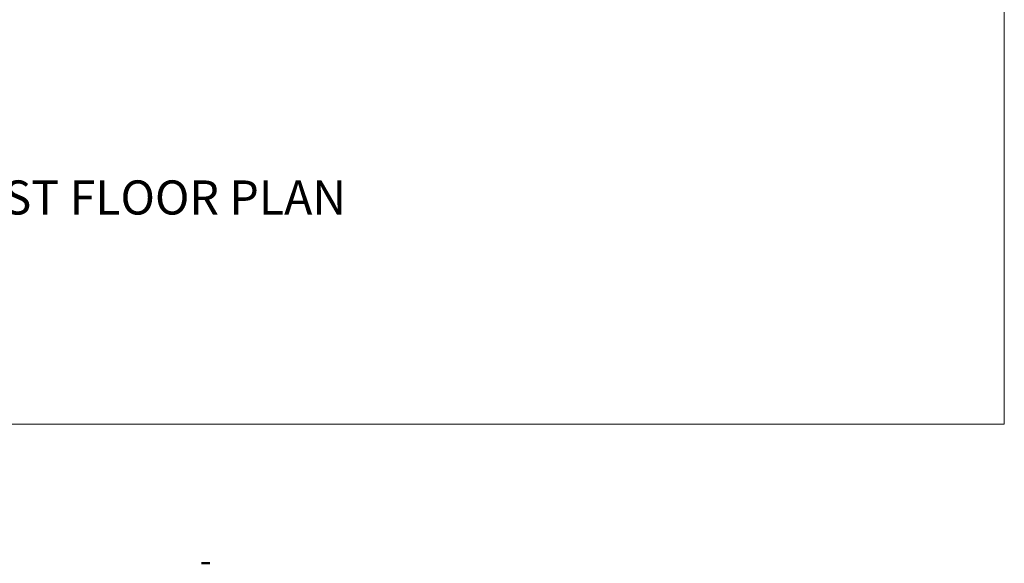
# Model space of a CAD drawing. Units: inches. Extents: x 1901 to 2863, y 888 to 2433.
# Tile 21 of 91: x 2343 to 2863, y 888 to 1175. Entities that reach past the tile are written whole.
import ezdxf

# ---------------------------------------------------------------- set-up
doc = ezdxf.new("R2010")
doc.units = ezdxf.units.IN
for name, color, linetype, lineweight in [('A-ANNO-TEXT', 7, 'Continuous', 35), ('A-FLOR-FIXT', 9, 'Continuous', 18), ('A-WALL', 7, 'Continuous', 50), ('A-WALL-PATT', 8, 'Continuous', 13)]:
    doc.layers.add(name, color=color, linetype=linetype, lineweight=lineweight)
doc.styles.get("Standard").update_dxf_attribs({"font": 'arial.ttf'})

msp = doc.modelspace()

# ---------------------------------------------------------------- hatches: boundary and pattern name
at = {"layer": 'A-WALL-PATT'}
h = msp.add_hatch(dxfattribs=at)
h.set_pattern_fill('ANSI32', color=256)
h.paths.add_polyline_path([(2192.5, 2274.13), (2141.26, 2274.13), (2141.26, 2269.63), (2192.5, 2269.63)])
h.paths.add_polyline_path([(2259.93, 2274.13), (2216.5, 2274.13), (2216.5, 2269.63), (2255.43, 2269.63), (2255.43, 2214.63), (2250.81, 2214.63), (2250.81, 2210.13), (2259.93, 2210.13), (2259.93, 2215.13), (2271.76, 2215.13), (2271.76, 2217.38), (2271.76, 2219.63), (2259.93, 2219.63)])
h.paths.add_polyline_path([(2171.43, 2269.63), (2166.93, 2269.63), (2166.93, 2219.63), (2121.24, 2219.63), (2121.24, 2215.13), (2166.93, 2215.13), (2166.93, 2083.13), (2161.81, 2083.13), (2161.81, 2078.63), (2171.43, 2078.63), (2177, 2078.63), (2177, 2080.88), (2177, 2083.13), (2171.43, 2083.13), (2171.43, 2210.13), (2230.91, 2210.13), (2230.91, 2212.38), (2230.91, 2214.63), (2171.43, 2214.63)])
h.paths.add_polyline_path([(2117.26, 2274.13), (2089.43, 2274.13), (2089.43, 2219.63), (2081.14, 2219.63), (2081.14, 2215.13), (2089.43, 2215.13), (2098, 2215.13), (2098, 2217.38), (2098, 2219.63), (2093.93, 2219.63), (2093.93, 2269.63), (2117.26, 2269.63), (2117.26, 2271.88)])
h.paths.add_polyline_path([(2343.43, 2219.63), (2329.29, 2219.63), (2329.29, 2215.13), (2338.93, 2215.13), (2338.93, 2184.74), (2343.43, 2184.74)])
h.paths.add_polyline_path([(2338.93, 2083.13), (2329.29, 2083.13), (2208.97, 2083.13), (2208.97, 2078.63), (2338.93, 2078.63)])
h.paths.add_polyline_path([(2343.43, 2136.74), (2338.93, 2136.74), (2338.93, 1872.63), (2343.43, 1872.63)])
h.paths.add_polyline_path([(2343.43, 1863.63), (2397.68, 1863.63), (2397.68, 1821.63), (2384.14, 1821.63), (2384.14, 1812.63), (2418.33, 1812.63), (2418.33, 1817.13), (2418.33, 1821.63), (2406.68, 1821.63), (2406.68, 1863.63), (2459.5, 1863.63), (2459.5, 1821.63), (2447.14, 1821.63), (2447.14, 1812.63), (2459.5, 1812.63), (2468.5, 1812.63), (2468.5, 1872.63), (2394.43, 1872.63), (2334.43, 1872.63), (2334.43, 1812.63), (2343.43, 1812.63), (2353.25, 1812.63), (2353.25, 1821.63), (2343.43, 1821.63)])
h.paths.add_polyline_path([(2510.01, 1872.63), (2468.5, 1872.63), (2468.5, 1868.13), (2510.01, 1868.13)])
h.paths.add_polyline_path([(2514.01, 1817.13), (2468.5, 1817.13), (2468.5, 1812.63), (2482.11, 1812.63), (2482.11, 1800.61), (2486.61, 1800.61), (2486.61, 1812.63), (2514.01, 1812.63)])
h.paths.add_polyline_path([(2299.25, 1814.88), (2299.25, 1817.13), (2295.93, 1817.13), (2295.93, 1854.17), (2293.68, 1854.17), (2291.43, 1854.17), (2291.43, 1817.13), (2266.11, 1817.13), (2266.11, 1812.63), (2299.25, 1812.63)])
h.paths.add_polyline_path([(2218.11, 1817.13), (2206.46, 1817.13), (2171.43, 1817.13), (2171.43, 1949.13), (2190.1, 1949.13), (2190.1, 1953.63), (2163.47, 1953.63), (2163.47, 1949.13), (2166.93, 1949.13), (2166.93, 1817.13), (2114.3, 1817.13), (2114.3, 1812.63), (2218.11, 1812.63)])
h.paths.add_polyline_path([(2029.43, 1970.92), (2024.93, 1970.92), (2024.93, 1912.72), (2029.43, 1912.72)])
h.paths.add_polyline_path([(2132.3, 1953.63), (2113.93, 1953.63), (2113.93, 1975.89), (2111.68, 1975.89), (2109.43, 1975.89), (2109.43, 1953.63), (2029.43, 1953.63), (2029.43, 1949.13), (2132.3, 1949.13)])
h.paths.add_polyline_path([(2029.43, 1853.61), (2029.31, 1853.61), (2029.31, 1853.61), (2029.43, 1853.61), (2029.43, 1864.72), (2024.93, 1864.72), (2024.93, 1812.63), (2066.3, 1812.63), (2066.3, 1814.88), (2066.3, 1817.13), (2029.43, 1817.13)])
h.paths.add_polyline_path([(2122.93, 2010.09), (2120.68, 2010.09), (2118.43, 2010.09), (2118.43, 2006.13), (2029.43, 2006.13), (2029.43, 2001.63), (2109.43, 2001.63), (2109.43, 1998.04), (2113.93, 1998.04), (2113.93, 2001.63), (2122.93, 2001.63)])
h.paths.add_polyline_path([(2029.43, 2031.38), (2024.93, 2031.38), (2024.93, 1994.92), (2027.18, 1994.92), (2029.43, 1994.92)])
h.paths.add_polyline_path([(2029.43, 2136.74), (2024.93, 2136.74), (2024.93, 2067.38), (2027.18, 2067.38), (2029.43, 2067.38)])
h.paths.add_polyline_path([(2125.62, 2083.13), (2029.43, 2083.13), (2029.43, 2078.63), (2118.43, 2078.63), (2118.43, 2030.71), (2122.93, 2030.71), (2122.93, 2078.63), (2125.62, 2078.63)])
h.paths.add_polyline_path([(2029.43, 2215.13), (2040.47, 2215.13), (2040.47, 2217.38), (2040.47, 2219.63), (2024.93, 2219.63), (2024.93, 2184.74), (2029.43, 2184.74), (2029.43, 2187.78)])
h.paths.add_polyline_path([(2686.43, 2274.13), (2659.28, 2274.13), (2659.28, 2269.63), (2681.93, 2269.63), (2681.93, 2219.63), (2676.82, 2219.63), (2676.82, 2215.13), (2681.93, 2215.13), (2697.01, 2215.13), (2697.01, 2217.38), (2697.01, 2219.63), (2686.43, 2219.63)])
h.paths.add_polyline_path([(2609.93, 2269.63), (2635.28, 2269.63), (2635.28, 2274.13), (2571.43, 2274.13), (2571.43, 2269.63), (2605.43, 2269.63), (2605.43, 2214.63), (2549.1, 2214.63), (2549.1, 2210.13), (2605.43, 2210.13), (2605.43, 2083.13), (2601.01, 2083.13), (2601.01, 2080.88), (2601.01, 2078.63), (2609.93, 2078.63), (2616.16, 2078.63), (2616.16, 2080.88), (2616.16, 2083.13), (2609.93, 2083.13), (2609.93, 2215.13), (2651.46, 2215.13), (2651.46, 2217.38), (2651.46, 2219.63), (2609.93, 2219.63)])
h.paths.add_polyline_path([(2521.43, 2269.63), (2547.43, 2269.63), (2547.43, 2271.88), (2547.43, 2274.13), (2516.93, 2274.13), (2516.93, 2219.63), (2506.41, 2219.63), (2506.41, 2215.13), (2516.93, 2215.13), (2516.93, 2210.13), (2525.4, 2210.13), (2525.4, 2212.38), (2525.4, 2214.63), (2521.43, 2214.63)])
h.paths.add_polyline_path([(2456.01, 2219.63), (2439.43, 2219.63), (2439.43, 2187.89), (2443.93, 2187.89), (2443.93, 2215.13), (2456.01, 2215.13)])
h.paths.add_polyline_path([(2752.93, 2219.63), (2739.48, 2219.63), (2739.48, 2215.13), (2748.43, 2215.13), (2748.43, 2187.89), (2752.93, 2187.89)])
h.paths.add_polyline_path([(2752.93, 2139.89), (2748.43, 2139.89), (2748.43, 2083.13), (2648.42, 2083.13), (2648.42, 2078.63), (2654.93, 2078.63), (2654.93, 2039.44), (2659.43, 2039.44), (2659.43, 2078.63), (2748.43, 2078.63), (2748.43, 2063.43), (2752.93, 2063.43)])
h.paths.add_polyline_path([(2752.93, 2010.63), (2659.43, 2010.63), (2659.43, 2015.65), (2654.93, 2015.65), (2654.93, 2010.63), (2605.43, 2010.63), (2605.43, 1920.97), (2609.93, 1920.97), (2609.93, 2006.13), (2748.43, 2006.13), (2748.43, 1982.47), (2752.93, 1982.47)])
h.paths.add_polyline_path([(2752.93, 2027.43), (2748.43, 2027.43), (2748.43, 2010.63), (2752.93, 2010.63)])
h.paths.add_polyline_path([(2748.43, 1886.13), (2609.93, 1886.13), (2609.93, 1889.72), (2605.43, 1889.72), (2605.43, 1861.26), (2609.93, 1861.26), (2609.93, 1881.63), (2748.43, 1881.63)])
h.paths.add_polyline_path([(2456.86, 2228.83), (2498.4, 2228.83), (2498.4, 2247.49), (2456.86, 2247.49)], flags=9)
h.paths.add_polyline_path([(2038.6, 2237.42), (2080.17, 2237.42), (2080.17, 2256.08), (2038.6, 2256.08)], flags=9)
h.paths.add_polyline_path([(2292.01, 1062.39), (2539.93, 1062.39), (2539.93, 1099.49), (2292.01, 1099.49)], flags=9)
h.paths.add_polyline_path([(2424.91, 1832.25), (2448.51, 1832.25), (2448.51, 1846.68), (2424.91, 1846.68)], flags=25)
h.paths.add_polyline_path([(2359.08, 1832.25), (2382.68, 1832.25), (2382.68, 1846.68), (2359.08, 1846.68)], flags=25)
h.paths.add_polyline_path([(2352.9, 1684.8), (2367.54, 1684.8), (2367.54, 1697.17), (2352.9, 1697.17)], flags=9)
h.paths.add_polyline_path([(2079.29, 1755.83), (2169.02, 1755.83), (2169.02, 1774.37), (2079.29, 1774.37)], flags=9)
h.paths.add_polyline_path([(2404.09, 1373.86), (2404.09, 1463.59), (2385.54, 1463.59), (2385.54, 1373.86)], flags=9)
h.paths.add_polyline_path([(2268.09, 2236.37), (2309.64, 2236.37), (2309.64, 2255.03), (2268.09, 2255.03)], flags=9)
h.paths.add_polyline_path([(2575.96, 1700.95), (2665.7, 1700.95), (2665.7, 1719.5), (2575.96, 1719.5)], flags=9)
h.paths.add_polyline_path([(2302.96, 1878.47), (2329.52, 1878.47), (2329.52, 1888.78), (2302.96, 1888.78)], flags=9)
h.paths.add_polyline_path([(2097.42, 2240.58), (2126.57, 2240.58), (2126.57, 2259.23), (2097.42, 2259.23)], flags=9)
h.paths.add_polyline_path([(2208.72, 2246.12), (2237.88, 2246.12), (2237.88, 2264.78), (2208.72, 2264.78)], flags=9)
h.paths.add_polyline_path([(2038.15, 1925.96), (2076.99, 1925.96), (2076.99, 1944.62), (2038.15, 1944.62)], flags=9)
h.paths.add_polyline_path([(2239.14, 1926.67), (2288.46, 1926.67), (2288.46, 1945.33), (2239.14, 1945.33)], flags=9)
h.paths.add_polyline_path([(2175.43, 2007.33), (2212.36, 2007.33), (2212.36, 2025.99), (2175.43, 2025.99)], flags=9)
h.paths.add_polyline_path([(2225.03, 2091.79), (2263.87, 2091.79), (2263.87, 2110.45), (2225.03, 2110.45)], flags=9)
h.paths.add_polyline_path([(2035.4, 2098.48), (2074.24, 2098.48), (2074.24, 2117.14), (2035.4, 2117.14)], flags=9)
h.paths.add_polyline_path([(2050.1, 2029.21), (2083.26, 2029.21), (2083.26, 2047.87), (2050.1, 2047.87)], flags=9)
h.paths.add_polyline_path([(2069.68, 1956.72), (2098.83, 1956.72), (2098.83, 1975.38), (2069.68, 1975.38)], flags=25)
h.paths.add_polyline_path([(2328.62, 1753.34), (2361.66, 1753.34), (2361.66, 1771.99), (2328.62, 1771.99)], flags=9)
h.paths.add_polyline_path([(2395.16, 2060.89), (2395.16, 2140.65), (2378.68, 2140.65), (2378.68, 2060.89)], flags=9)
h.paths.add_polyline_path([(2463.73, 2059.02), (2492.89, 2059.02), (2492.89, 2077.68), (2463.73, 2077.68)], flags=9)
h.paths.add_polyline_path([(2458.03, 2181.54), (2496.87, 2181.54), (2496.87, 2200.19), (2458.03, 2200.19)], flags=9)
h.paths.add_polyline_path([(2527.58, 2243.07), (2556.73, 2243.07), (2556.73, 2261.73), (2527.58, 2261.73)], flags=9)
h.paths.add_polyline_path([(2694.46, 2232.77), (2736.03, 2232.77), (2736.03, 2251.42), (2694.46, 2251.42)], flags=9)
h.paths.add_polyline_path([(2637.82, 2249.22), (2666.98, 2249.22), (2666.98, 2267.88), (2637.82, 2267.88)], flags=9)
h.paths.add_polyline_path([(2623.69, 2183.54), (2662.53, 2183.54), (2662.53, 2202.2), (2623.69, 2202.2)], flags=9)
h.paths.add_polyline_path([(2691.97, 2021.5), (2725.12, 2021.5), (2725.12, 2040.16), (2691.97, 2040.16)], flags=9)
h.paths.add_polyline_path([(2621.04, 1975.91), (2662.34, 1975.91), (2662.34, 1994.57), (2621.04, 1994.57)], flags=25)
h.paths.add_polyline_path([(2479.03, 1927.62), (2519.84, 1927.62), (2519.84, 1946.28), (2479.03, 1946.28)], flags=9)
h.paths.add_polyline_path([(2670.94, 1849.08), (2716.01, 1849.08), (2716.01, 1867.73), (2670.94, 1867.73)], flags=9)
h.paths.add_polyline_path([(2523.61, 1782.96), (2550.17, 1782.96), (2550.17, 1793.26), (2523.61, 1793.26)], flags=9)
h.paths.add_polyline_path([(2450.84, 1207.33), (2492.39, 1207.33), (2492.39, 1225.99), (2450.84, 1225.99)], flags=9)
h.paths.add_polyline_path([(2527.75, 1203.84), (2556.91, 1203.84), (2556.91, 1222.5), (2527.75, 1222.5)], flags=9)
h.paths.add_polyline_path([(2639.11, 1207.2), (2668.27, 1207.2), (2668.27, 1225.86), (2639.11, 1225.86)], flags=9)
h.paths.add_polyline_path([(2692.59, 1218.97), (2734.17, 1218.97), (2734.17, 1237.62), (2692.59, 1237.62)], flags=9)
h.paths.add_polyline_path([(2669.27, 1366.33), (2708.11, 1366.33), (2708.11, 1384.99), (2669.27, 1384.99)], flags=9)
h.paths.add_polyline_path([(2463.31, 1358.03), (2502.15, 1358.03), (2502.15, 1376.69), (2463.31, 1376.69)], flags=9)
h.paths.add_polyline_path([(2494.72, 1449.96), (2531.65, 1449.96), (2531.65, 1468.62), (2494.72, 1468.62)], flags=9)
h.paths.add_polyline_path([(2675.57, 1422.16), (2708.72, 1422.16), (2708.72, 1440.81), (2675.57, 1440.81)], flags=9)
h.paths.add_polyline_path([(2685.63, 1493.89), (2714.79, 1493.89), (2714.79, 1512.55), (2685.63, 1512.55)], flags=9)
h.paths.add_polyline_path([(2686.8, 1529.91), (2725.65, 1529.91), (2725.65, 1548.57), (2686.8, 1548.57)], flags=9)
h.paths.add_polyline_path([(2503.65, 1537.99), (2552.97, 1537.99), (2552.97, 1556.65), (2503.65, 1556.65)], flags=9)
h.paths.add_polyline_path([(2291.71, 1643.5), (2318.28, 1643.5), (2318.28, 1653.81), (2291.71, 1653.81)], flags=9)
h.paths.add_polyline_path([(2450.63, 1610.52), (2477.19, 1610.52), (2477.19, 1620.82), (2450.63, 1620.82)], flags=9)
h.paths.add_polyline_path([(2359.99, 1551.81), (2422.25, 1551.81), (2422.25, 1562.12), (2359.99, 1562.12)], flags=9)
h.paths.add_polyline_path([(2280.11, 1249.01), (2321.65, 1249.01), (2321.65, 1267.66), (2280.11, 1267.66)], flags=9)
h.paths.add_polyline_path([(2164.06, 1274.23), (2193.22, 1274.23), (2193.22, 1292.89), (2164.06, 1292.89)], flags=9)
h.paths.add_polyline_path([(2118.21, 1277.69), (2151.25, 1277.69), (2151.25, 1296.35), (2118.21, 1296.35)], flags=9)
h.paths.add_polyline_path([(2031.95, 1268.53), (2073.52, 1268.53), (2073.52, 1287.19), (2031.95, 1287.19)], flags=9)
h.paths.add_polyline_path([(2050.2, 1409.08), (2089.04, 1409.08), (2089.04, 1427.74), (2050.2, 1427.74)], flags=9)
h.paths.add_polyline_path([(2243.74, 1421.03), (2282.58, 1421.03), (2282.58, 1439.69), (2243.74, 1439.69)], flags=9)
h.paths.add_polyline_path([(2190.75, 1509.77), (2231.56, 1509.77), (2231.56, 1528.43), (2190.75, 1528.43)], flags=9)
h.paths.add_polyline_path([(2058.39, 1475.42), (2091.55, 1475.42), (2091.55, 1494.07), (2058.39, 1494.07)], flags=9)
h.paths.add_polyline_path([(2062.45, 1553.09), (2091.6, 1553.09), (2091.6, 1571.75), (2062.45, 1571.75)], flags=9)
h.paths.add_polyline_path([(2219.52, 1590.37), (2266.15, 1590.37), (2266.15, 1609.02), (2219.52, 1609.02)], flags=9)
h.paths.add_polyline_path([(2041.07, 1584.19), (2079.91, 1584.19), (2079.91, 1602.85), (2041.07, 1602.85)], flags=9)
h = msp.add_hatch(dxfattribs=at)
h.set_pattern_fill('ANSI32', color=256)
h.paths.add_polyline_path([(2443.93, 2139.89), (2439.43, 2139.89), (2439.43, 2069.35), (2441.68, 2069.35), (2443.93, 2069.35), (2443.93, 2078.63), (2521.93, 2078.63), (2521.93, 2075.07), (2524.18, 2075.07), (2526.43, 2075.07), (2526.43, 2078.63), (2571.75, 2078.63), (2571.75, 2080.88), (2571.75, 2083.13), (2443.93, 2083.13)])
h.paths.add_polyline_path([(2526.43, 2054.63), (2524.18, 2054.63), (2521.93, 2054.63), (2521.93, 2030.63), (2443.93, 2030.63), (2443.93, 2045.35), (2439.43, 2045.35), (2439.43, 1983.87), (2443.93, 1983.87), (2443.93, 2026.13), (2521.93, 2026.13), (2526.43, 2026.13)])
h.paths.add_polyline_path([(2443.93, 1923.87), (2439.43, 1923.87), (2439.43, 1872.63), (2443.93, 1872.63)])
h.paths.add_polyline_path([(2636.23, 1766.13), (2609.93, 1766.13), (2609.93, 1779.79), (2605.43, 1779.79), (2605.43, 1766.13), (2486.61, 1766.13), (2486.61, 1770.67), (2482.11, 1770.67), (2482.11, 1766.13), (2482.11, 1761.63), (2636.23, 1761.63), (2636.23, 1763.88)])
h.paths.add_polyline_path([(2519.54, 1663.38), (2519.54, 1665.63), (2494.93, 1665.63), (2481.83, 1665.63), (2481.83, 1663.38), (2481.83, 1661.13), (2490.43, 1661.13), (2490.43, 1640.16), (2494.93, 1640.16), (2494.93, 1661.13), (2519.54, 1661.13)])
h.paths.add_polyline_path([(2443.93, 1712.13), (2443.93, 1716.63), (2414.46, 1716.63), (2414.46, 1712.13), (2439.43, 1712.13), (2439.43, 1545.51), (2443.93, 1545.51), (2443.93, 1661.13), (2448.47, 1661.13), (2448.47, 1665.63), (2443.93, 1665.63)])
h.paths.add_polyline_path([(2343.43, 1712.13), (2365.52, 1712.13), (2365.52, 1714.38), (2365.52, 1716.63), (2333.87, 1716.63), (2333.87, 1714.38), (2333.87, 1712.13), (2338.93, 1712.13), (2338.93, 1575.63), (2338.93, 1545.51), (2343.43, 1545.51), (2343.43, 1547.51), (2343.43, 1580.13)])
h.paths.add_polyline_path([(2752.93, 1665.63), (2579.54, 1665.63), (2579.54, 1661.13), (2615.93, 1661.13), (2615.93, 1529.13), (2598.93, 1529.13), (2598.93, 1524.63), (2623.13, 1524.63), (2623.13, 1526.88), (2623.13, 1529.13), (2620.43, 1529.13), (2620.43, 1661.13), (2748.43, 1661.13), (2748.43, 1633.5), (2752.93, 1633.5)])
h.paths.add_polyline_path([(2752.93, 1419.93), (2748.43, 1419.93), (2748.43, 1400.13), (2659.43, 1400.13), (2659.43, 1444.33), (2657.18, 1444.33), (2654.93, 1444.33), (2654.93, 1400.13), (2643.65, 1400.13), (2643.65, 1395.63), (2748.43, 1395.63), (2748.43, 1364.04), (2752.93, 1364.04)])
h.paths.add_polyline_path([(2752.93, 1492.88), (2748.43, 1492.88), (2748.43, 1476.63), (2667.43, 1476.63), (2667.43, 1479.71), (2665.18, 1479.71), (2662.93, 1479.71), (2662.93, 1476.63), (2654.93, 1476.63), (2654.93, 1469.54), (2659.43, 1469.54), (2659.43, 1472.13), (2748.43, 1472.13), (2748.43, 1455.93), (2752.93, 1455.93)])
h.paths.add_polyline_path([(2752.93, 1304.04), (2748.43, 1304.04), (2748.43, 1263.63), (2738.66, 1263.63), (2738.66, 1259.13), (2752.93, 1259.13)])
h.paths.add_polyline_path([(2685.93, 1259.13), (2695.49, 1259.13), (2695.49, 1261.38), (2695.49, 1263.63), (2677.84, 1263.63), (2677.84, 1261.38), (2677.84, 1259.13), (2681.43, 1259.13), (2681.43, 1203.63), (2653.28, 1203.63), (2653.28, 1199.13), (2685.93, 1199.13), (2685.93, 1203.63)])
h.paths.add_polyline_path([(2609.43, 1395.63), (2611.85, 1395.63), (2611.85, 1400.13), (2598.89, 1400.13), (2598.89, 1397.88), (2598.89, 1395.63), (2604.93, 1395.63), (2604.93, 1268.13), (2554.73, 1268.13), (2554.73, 1265.88), (2554.73, 1263.63), (2604.93, 1263.63), (2604.93, 1203.63), (2571.31, 1203.63), (2571.31, 1199.13), (2604.93, 1199.13), (2629.28, 1199.13), (2629.28, 1201.38), (2629.28, 1203.63), (2609.43, 1203.63), (2609.43, 1258.63), (2609.43, 1259.13), (2654.8, 1259.13), (2654.8, 1263.63), (2609.43, 1263.63)])
h.paths.add_polyline_path([(2443.93, 1304.04), (2439.43, 1304.04), (2439.43, 1259.13), (2443.93, 1259.13), (2456.16, 1259.13), (2456.16, 1261.38), (2456.16, 1263.63), (2443.93, 1263.63)])
h.paths.add_polyline_path([(2525.43, 1263.63), (2531.78, 1263.63), (2531.78, 1268.13), (2520.93, 1268.13), (2520.93, 1263.63), (2511.41, 1263.63), (2511.41, 1259.13), (2520.93, 1259.13), (2520.93, 1199.13), (2547.31, 1199.13), (2547.31, 1201.38), (2547.31, 1203.63), (2525.43, 1203.63)])
h.paths.add_polyline_path([(2443.93, 1434.84), (2439.43, 1434.84), (2439.43, 1364.04), (2441.68, 1364.04), (2443.93, 1364.04)])
h.paths.add_polyline_path([(2567.13, 1400.13), (2443.93, 1400.13), (2443.93, 1395.63), (2567.13, 1395.63)])
h.paths.add_polyline_path([(2443.93, 1545.51), (2439.43, 1545.51), (2439.43, 1494.84), (2443.93, 1494.84)])
h.paths.add_polyline_path([(2494.93, 1553.35), (2492.68, 1553.35), (2490.43, 1553.35), (2490.43, 1524.63), (2494.93, 1524.63), (2525.94, 1524.63), (2525.94, 1526.88), (2525.94, 1529.13), (2494.93, 1529.13)])
h.paths.add_polyline_path([(2752.93, 1573.5), (2748.43, 1573.5), (2748.43, 1529.13), (2657.76, 1529.13), (2657.76, 1524.63), (2662.93, 1524.63), (2662.93, 1498.63), (2667.43, 1498.63), (2667.43, 1524.63), (2748.43, 1524.63), (2748.43, 1516.88), (2752.93, 1516.88)])
h.paths.add_polyline_path([(2038.6, 2237.42), (2080.17, 2237.42), (2080.17, 2256.08), (2038.6, 2256.08)], flags=9)
h.paths.add_polyline_path([(2292.01, 1062.39), (2539.93, 1062.39), (2539.93, 1099.49), (2292.01, 1099.49)], flags=9)
h.paths.add_polyline_path([(2424.91, 1832.25), (2448.51, 1832.25), (2448.51, 1846.68), (2424.91, 1846.68)], flags=9)
h.paths.add_polyline_path([(2359.08, 1832.25), (2382.68, 1832.25), (2382.68, 1846.68), (2359.08, 1846.68)], flags=9)
h.paths.add_polyline_path([(2352.9, 1684.8), (2367.54, 1684.8), (2367.54, 1697.17), (2352.9, 1697.17)], flags=9)
h.paths.add_polyline_path([(2079.29, 1755.83), (2169.02, 1755.83), (2169.02, 1774.37), (2079.29, 1774.37)], flags=9)
h.paths.add_polyline_path([(2404.09, 1373.86), (2404.09, 1463.59), (2385.54, 1463.59), (2385.54, 1373.86)], flags=9)
h.paths.add_polyline_path([(2268.09, 2236.37), (2309.64, 2236.37), (2309.64, 2255.03), (2268.09, 2255.03)], flags=9)
h.paths.add_polyline_path([(2575.96, 1700.95), (2665.7, 1700.95), (2665.7, 1719.5), (2575.96, 1719.5)], flags=9)
h.paths.add_polyline_path([(2302.96, 1878.47), (2329.52, 1878.47), (2329.52, 1888.78), (2302.96, 1888.78)], flags=9)
h.paths.add_polyline_path([(2097.42, 2240.58), (2126.57, 2240.58), (2126.57, 2259.23), (2097.42, 2259.23)], flags=9)
h.paths.add_polyline_path([(2208.72, 2246.12), (2237.88, 2246.12), (2237.88, 2264.78), (2208.72, 2264.78)], flags=9)
h.paths.add_polyline_path([(2038.15, 1925.96), (2076.99, 1925.96), (2076.99, 1944.62), (2038.15, 1944.62)], flags=9)
h.paths.add_polyline_path([(2239.14, 1926.67), (2288.46, 1926.67), (2288.46, 1945.33), (2239.14, 1945.33)], flags=9)
h.paths.add_polyline_path([(2175.43, 2007.33), (2212.36, 2007.33), (2212.36, 2025.99), (2175.43, 2025.99)], flags=9)
h.paths.add_polyline_path([(2225.03, 2091.79), (2263.87, 2091.79), (2263.87, 2110.45), (2225.03, 2110.45)], flags=9)
h.paths.add_polyline_path([(2035.4, 2098.48), (2074.24, 2098.48), (2074.24, 2117.14), (2035.4, 2117.14)], flags=9)
h.paths.add_polyline_path([(2050.1, 2029.21), (2083.26, 2029.21), (2083.26, 2047.87), (2050.1, 2047.87)], flags=9)
h.paths.add_polyline_path([(2069.68, 1956.72), (2098.83, 1956.72), (2098.83, 1975.38), (2069.68, 1975.38)], flags=9)
h.paths.add_polyline_path([(2328.62, 1753.34), (2361.66, 1753.34), (2361.66, 1771.99), (2328.62, 1771.99)], flags=9)
h.paths.add_polyline_path([(2395.16, 2060.89), (2395.16, 2140.65), (2378.68, 2140.65), (2378.68, 2060.89)], flags=9)
h.paths.add_polyline_path([(2463.73, 2059.02), (2492.89, 2059.02), (2492.89, 2077.68), (2463.73, 2077.68)], flags=9)
h.paths.add_polyline_path([(2458.03, 2181.54), (2496.87, 2181.54), (2496.87, 2200.19), (2458.03, 2200.19)], flags=9)
h.paths.add_polyline_path([(2456.86, 2228.83), (2498.4, 2228.83), (2498.4, 2247.49), (2456.86, 2247.49)], flags=9)
h.paths.add_polyline_path([(2527.58, 2243.07), (2556.73, 2243.07), (2556.73, 2261.73), (2527.58, 2261.73)], flags=9)
h.paths.add_polyline_path([(2694.46, 2232.77), (2736.03, 2232.77), (2736.03, 2251.42), (2694.46, 2251.42)], flags=9)
h.paths.add_polyline_path([(2637.82, 2249.22), (2666.98, 2249.22), (2666.98, 2267.88), (2637.82, 2267.88)], flags=9)
h.paths.add_polyline_path([(2623.69, 2183.54), (2662.53, 2183.54), (2662.53, 2202.2), (2623.69, 2202.2)], flags=9)
h.paths.add_polyline_path([(2691.97, 2021.5), (2725.12, 2021.5), (2725.12, 2040.16), (2691.97, 2040.16)], flags=9)
h.paths.add_polyline_path([(2621.04, 1975.91), (2662.34, 1975.91), (2662.34, 1994.57), (2621.04, 1994.57)], flags=9)
h.paths.add_polyline_path([(2479.03, 1927.62), (2519.84, 1927.62), (2519.84, 1946.28), (2479.03, 1946.28)], flags=9)
h.paths.add_polyline_path([(2670.94, 1849.08), (2716.01, 1849.08), (2716.01, 1867.73), (2670.94, 1867.73)], flags=9)
h.paths.add_polyline_path([(2523.61, 1782.96), (2550.17, 1782.96), (2550.17, 1793.26), (2523.61, 1793.26)], flags=9)
h.paths.add_polyline_path([(2450.84, 1207.33), (2492.39, 1207.33), (2492.39, 1225.99), (2450.84, 1225.99)], flags=9)
h.paths.add_polyline_path([(2527.75, 1203.84), (2556.91, 1203.84), (2556.91, 1222.5), (2527.75, 1222.5)], flags=9)
h.paths.add_polyline_path([(2639.11, 1207.2), (2668.27, 1207.2), (2668.27, 1225.86), (2639.11, 1225.86)], flags=9)
h.paths.add_polyline_path([(2692.59, 1218.97), (2734.17, 1218.97), (2734.17, 1237.62), (2692.59, 1237.62)], flags=9)
h.paths.add_polyline_path([(2669.27, 1366.33), (2708.11, 1366.33), (2708.11, 1384.99), (2669.27, 1384.99)], flags=25)
h.paths.add_polyline_path([(2463.31, 1358.03), (2502.15, 1358.03), (2502.15, 1376.69), (2463.31, 1376.69)], flags=9)
h.paths.add_polyline_path([(2494.72, 1449.96), (2531.65, 1449.96), (2531.65, 1468.62), (2494.72, 1468.62)], flags=9)
h.paths.add_polyline_path([(2675.57, 1422.16), (2708.72, 1422.16), (2708.72, 1440.81), (2675.57, 1440.81)], flags=25)
h.paths.add_polyline_path([(2685.63, 1493.89), (2714.79, 1493.89), (2714.79, 1512.55), (2685.63, 1512.55)], flags=9)
h.paths.add_polyline_path([(2686.8, 1529.91), (2725.65, 1529.91), (2725.65, 1548.57), (2686.8, 1548.57)], flags=25)
h.paths.add_polyline_path([(2503.65, 1537.99), (2552.97, 1537.99), (2552.97, 1556.65), (2503.65, 1556.65)], flags=9)
h.paths.add_polyline_path([(2291.71, 1643.5), (2318.28, 1643.5), (2318.28, 1653.81), (2291.71, 1653.81)], flags=9)
h.paths.add_polyline_path([(2450.63, 1610.52), (2477.19, 1610.52), (2477.19, 1620.82), (2450.63, 1620.82)], flags=9)
h.paths.add_polyline_path([(2359.99, 1551.81), (2422.25, 1551.81), (2422.25, 1562.12), (2359.99, 1562.12)], flags=9)
h.paths.add_polyline_path([(2280.11, 1249.01), (2321.65, 1249.01), (2321.65, 1267.66), (2280.11, 1267.66)], flags=9)
h.paths.add_polyline_path([(2164.06, 1274.23), (2193.22, 1274.23), (2193.22, 1292.89), (2164.06, 1292.89)], flags=9)
h.paths.add_polyline_path([(2118.21, 1277.69), (2151.25, 1277.69), (2151.25, 1296.35), (2118.21, 1296.35)], flags=9)
h.paths.add_polyline_path([(2031.95, 1268.53), (2073.52, 1268.53), (2073.52, 1287.19), (2031.95, 1287.19)], flags=9)
h.paths.add_polyline_path([(2050.2, 1409.08), (2089.04, 1409.08), (2089.04, 1427.74), (2050.2, 1427.74)], flags=9)
h.paths.add_polyline_path([(2243.74, 1421.03), (2282.58, 1421.03), (2282.58, 1439.69), (2243.74, 1439.69)], flags=9)
h.paths.add_polyline_path([(2190.75, 1509.77), (2231.56, 1509.77), (2231.56, 1528.43), (2190.75, 1528.43)], flags=9)
h.paths.add_polyline_path([(2058.39, 1475.42), (2091.55, 1475.42), (2091.55, 1494.07), (2058.39, 1494.07)], flags=9)
h.paths.add_polyline_path([(2062.45, 1553.09), (2091.6, 1553.09), (2091.6, 1571.75), (2062.45, 1571.75)], flags=9)
h.paths.add_polyline_path([(2219.52, 1590.37), (2266.15, 1590.37), (2266.15, 1609.02), (2219.52, 1609.02)], flags=9)
h.paths.add_polyline_path([(2041.07, 1584.19), (2079.91, 1584.19), (2079.91, 1602.85), (2041.07, 1602.85)], flags=9)

# ---------------------------------------------------------------- linework, layer by layer
at = {"layer": 'A-FLOR-FIXT'}
msp.add_lwpolyline([(1901.45, 2433.12), (2863.43, 2433.12), (2863.43, 961.82), (1901.45, 961.82)], close=True, dxfattribs=at)
at = {"layer": 'A-WALL'}
msp.add_line((2443.93, 888.42), (2439.43, 888.42), dxfattribs=at)

# ---------------------------------------------------------------- texts
at = {"layer": 'A-ANNO-TEXT', "insert": (2298.57, 1090.54), "char_height": 18, "attachment_point": 1}
msp.add_mtext_dynamic_manual_height_columns('FIRST FLOOR PLAN', width=549.622, gutter_width=12.5, heights=[0], dxfattribs=at)

doc.saveas('drawing.dxf')
